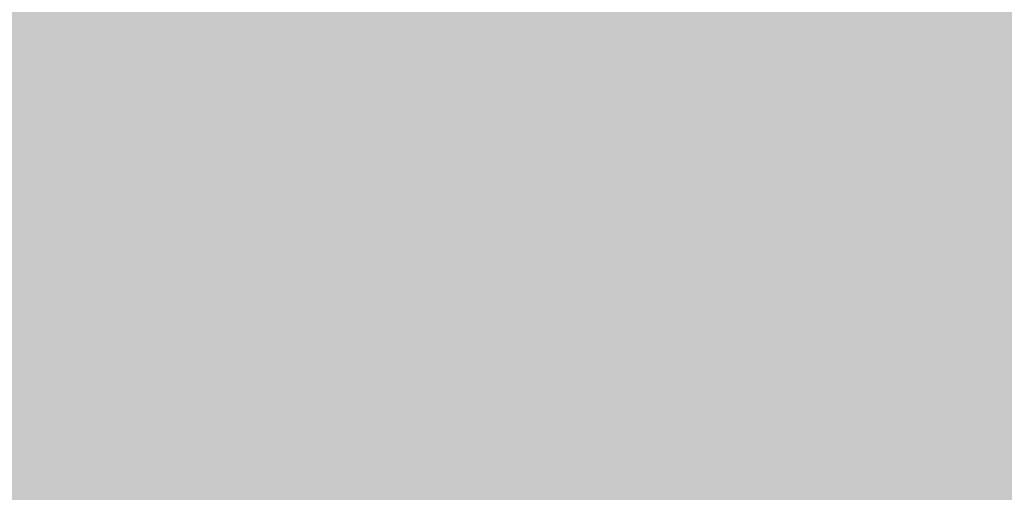
# Model space of a CAD drawing. Units: inches. Extents: x 2083 to 3317, y 1141 to 2115.
# Tile 136 of 256: x 3123.979 to 3126.132, y 1264.131 to 1265.165. Entities that reach past the tile are written whole.
import ezdxf

# ---------------------------------------------------------------- set-up
doc = ezdxf.new("R2010")
doc.units = ezdxf.units.IN
doc.layers.add('A-ANNO-DIMS', color=2, linetype='Continuous', lineweight=18)
doc.layers.add('A-WALL-PATT', color=251, linetype='Continuous', lineweight=13, true_color=0x636466)
doc.styles.get("Standard").update_dxf_attribs({"font": 'arial.ttf'})
doc.dimstyles.new('ISO-25', dxfattribs={"dimtxt": 12, "dimasz": 12, "dimexe": 1.25, "dimexo": 0.625, "dimtad": 1, "dimlunit": 3, "dimtxsty": 'Standard', "dimcen": 2.5, "dimadec": 0, "dimazin": 0, "dimtfac": 1, "dimtmove": 0, "dimatfit": 3, "dimfxl": 1, "dimarcsym": 0})

# ---------------------------------------------------------------- blocks, each defined once
blk = doc.blocks.new('*D26')
at = {"layer": 'A-ANNO-DIMS', "color": 0, "lineweight": -2, "transparency": 16777216}
for p, q in [((3088.9858, 1274.9151), (3088.9858, 1270.952)), ((3111.24, 1274.9151), (3111.24, 1270.952)), ((3076.9858, 1272.202), (2840.2624, 1272.202)), ((3111.24, 1272.202), (3088.9858, 1272.202)), ((3123.24, 1272.202), (3135.24, 1272.202))]:
    blk.add_line(p, q, dxfattribs=at)
at = {"layer": 'A-ANNO-DIMS', "color": 0, "transparency": 16777216}
for points in [[(3076.9858, 1274.202), (3076.9858, 1270.202), (3088.9858, 1272.202)], [(3123.24, 1274.202), (3123.24, 1270.202), (3111.24, 1272.202)]]:
    blk.add_solid(points, dxfattribs=at)
at = {"layer": 'Defpoints', "color": 0, "transparency": 16777216}
for p in [(3088.9858, 1275.5401), (3111.24, 1275.5401), (3088.9858, 1272.202)]:
    blk.add_point(p, dxfattribs=at)
at = {"layer": 'A-ANNO-DIMS', "color": 0, "transparency": 16777216, "insert": (2952.6241, 1279.0316), "char_height": 12, "attachment_point": 5}
blk.add_mtext('NIGHTSTAND 1\'-10 1/2" TYP.', dxfattribs=at)
blk = doc.blocks.new('*D27')
at = {"layer": 'A-ANNO-DIMS', "color": 0, "lineweight": -2, "transparency": 16777216}
for p, q in [((3114.5782, 1309.7943), (3114.5782, 1321.7943)), ((3111.865, 1297.7943), (3115.8282, 1297.7943)), ((3114.5782, 1297.7943), (3114.5782, 1275.5401)), ((3111.865, 1275.5401), (3115.8282, 1275.5401)), ((3114.5782, 1263.5401), (3114.5782, 1140.9886))]:
    blk.add_line(p, q, dxfattribs=at)
at = {"layer": 'A-ANNO-DIMS', "color": 0, "transparency": 16777216}
for points in [[(3112.5782, 1309.7943), (3116.5782, 1309.7943), (3114.5782, 1297.7943)], [(3112.5782, 1263.5401), (3116.5782, 1263.5401), (3114.5782, 1275.5401)]]:
    blk.add_solid(points, dxfattribs=at)
at = {"layer": 'Defpoints', "color": 0, "transparency": 16777216}
for p in [(3111.24, 1297.7943), (3111.24, 1275.5401), (3114.5782, 1275.5401)]:
    blk.add_point(p, dxfattribs=at)
at = {"layer": 'A-ANNO-DIMS', "color": 0, "transparency": 16777216, "insert": (3107.7485, 1196.2643), "char_height": 12, "attachment_point": 5, "rotation": 90}
blk.add_mtext('1\'-10 1/2" TYP.', dxfattribs=at)

msp = doc.modelspace()

# ---------------------------------------------------------------- hatches: boundary and pattern name
at = {"layer": 'A-WALL-PATT'}
h = msp.add_hatch(color=256, dxfattribs=at)
h.dxf.hatch_style = 1
h.paths.add_polyline_path([(3126.9598, 2020.7614), (2748.9598, 2020.7614), (2604.9598, 2020.7614), (2226.9598, 2020.7614), (2226.9598, 1702.7614), (2466.9598, 1702.7614), (2466.9598, 1582.7614), (2418.9598, 1582.7614), (2418.9598, 1477.7614), (2226.9598, 1477.7614), (2226.9598, 1263.2614), (2544.9598, 1263.2614), (2544.9598, 1411.7614), (2604.9598, 1411.7614), (2685.9598, 1411.7614), (2685.9598, 1420.7614), (2604.9598, 1420.7614), (2604.9598, 1573.7614), (2604.9598, 1702.7614), (2604.9598, 2011.7614), (2748.9598, 2011.7614), (2748.9598, 1702.7614), (2862.9598, 1702.7614), (2862.9598, 1621.7614), (2871.9598, 1621.7614), (2871.9598, 1702.7614), (2883.9598, 1702.7614), (2883.9598, 1706.9395, -0.026459), (2883.9598, 1711.7614), (2757.9598, 1711.7614), (2757.9598, 1807.7614), (2787.9598, 1807.7614), (2787.9598, 1812.2614), (2757.9598, 1812.2614), (2757.9598, 2011.7614), (2877.9598, 2011.7614), (2877.9598, 1812.2614), (2847.9598, 1812.2614), (2847.9598, 1807.7614), (2889.8357, 1807.7614), (2889.8357, 1812.2614), (2882.4598, 1812.2614), (2882.4598, 2011.7614), (3117.9598, 2011.7614), (3117.9598, 1812.2614), (2937.8357, 1812.2614), (2937.8357, 1807.7614), (2995.7098, 1807.7614), (2995.7098, 1796.1177), (3000.2098, 1796.1177), (3000.2098, 1807.7614), (3117.9598, 1807.7614), (3117.9598, 1711.7614), (3000.2098, 1711.7614), (3000.2098, 1760.1177), (2998.5727, 1760.1177, -0.020711), (2995.7098, 1760.1177), (2995.7098, 1711.7614), (2931.9598, 1711.7614), (2931.9598, 1702.7614), (3126.9598, 1702.7614)])
h.paths.add_polyline_path([(2471.4598, 2011.7614), (2471.4598, 1810.0114), (2462.7169, 1810.0114), (2462.7169, 1805.5114), (2505.9598, 1805.5114), (2505.9598, 1810.0114), (2475.9598, 1810.0114), (2475.9598, 2011.7614), (2595.9598, 2011.7614), (2595.9598, 1810.0114), (2565.9598, 1810.0114), (2565.9598, 1805.5114), (2595.9598, 1805.5114), (2595.9598, 1711.7614), (2235.9598, 1711.7614), (2235.9598, 1805.5114), (2353.7098, 1805.5114), (2353.7098, 1796.0542), (2358.2098, 1796.0542), (2358.2098, 1805.5114), (2414.7169, 1805.5114), (2414.7169, 1810.0114), (2235.9598, 1810.0114), (2235.9598, 2011.7614)], flags=16)
h.paths.add_polyline_path([(2270.2047, 1994.61), (2270.2047, 1970.61), (2246.2047, 1970.61), (2246.2047, 1994.61)], flags=0)
edge = h.paths.add_edge_path(flags=0)
edge.add_ellipse((2332.0274, 1899.7982), major_axis=(-3.043, 3.043), ratio=0.168252, start_angle=-161.3322, end_angle=-156.3071, ccw=False)
edge.add_ellipse((2333.082, 1898.7435), major_axis=(-1.0546, 1.0546), ratio=0.453532, start_angle=-123.371, end_angle=-94.1591)
edge = h.paths.add_edge_path(flags=0)
edge.add_ellipse((2332.0274, 1968.8763), major_axis=(3.043, 3.043), ratio=0.168252, start_angle=18.6678, end_angle=23.6929)
edge.add_spline(control_points=[(2332.9256, 1970.6911), (2332.2268, 1970.3361), (2330.8937, 1969.6589), (2328.4131, 1970.9321), (2327.2039, 1967.7487), (2324.7096, 1969.9556), (2322.5328, 1967.0124), (2320.0128, 1971.2958), (2317.6803, 1968.1578), (2316.0405, 1967.102), (2315.4269, 1966.8096)], knot_values=[0, 0, 0, 0, 2.267059, 4.324559, 6.685584, 8.878641, 11.121502, 14.300359, 17.755284, 19.732645, 19.732645, 19.732645, 19.732645], degree=3, periodic=0)
edge.add_ellipse((2332.0274, 1968.8763), major_axis=(3.043, 3.043), ratio=0.168252, start_angle=18.6678, end_angle=23.6929, ccw=False)
edge.add_ellipse((2333.082, 1969.9309), major_axis=(1.0546, 1.0546), ratio=0.453532, start_angle=56.629, end_angle=85.8409, ccw=False)
edge = h.paths.add_edge_path(flags=0)
edge.add_spline(control_points=[(2296.4283, 1967.9879), (2293.6278, 1965.3363), (2287.7036, 1959.7271), (2299.7439, 1949.9957), (2294.5326, 1935.6685), (2290.5732, 1920.6035), (2293.3941, 1909.9737), (2296.1854, 1904.9665)], knot_values=[0.099185, 0.099185, 0.099185, 0.099185, 0.345301, 0.619822, 0.982653, 1.386093, 1.810555, 1.810555, 1.810555, 1.810555], degree=3, periodic=0)
edge.add_spline(control_points=[(2296.1854, 1904.9665), (2297.3836, 1902.6193), (2298.001, 1901.9493), (2298.553, 1901.4682)], knot_values=[0.006246, 0.006246, 0.006246, 0.006246, 0.055476, 0.055476, 0.055476, 0.055476], degree=3, periodic=0)
edge.add_spline(control_points=[(2298.553, 1901.4682), (2297.2586, 1900.9232), (2295.2253, 1900.2321), (2293.0602, 1900.6142), (2292.1014, 1900.7884), (2292.0896, 1900.7906)], knot_values=[0.312835, 0.312835, 0.312835, 0.312835, 0.40178, 0.474987, 0.475903, 0.475903, 0.475903, 0.475903], degree=3, periodic=0)
edge.add_arc((2292.7936, 1904.6641), 3.937, 215.4209, 259.6982, ccw=False)
edge.add_spline(control_points=[(2289.5853, 1902.3823), (2289.4767, 1902.5351), (2289.3685, 1902.688), (2289.2609, 1902.8412)], knot_values=[0.102872, 0.102872, 0.102872, 0.102872, 0.116896, 0.116896, 0.116896, 0.116896], degree=3, periodic=0)
edge.add_spline(control_points=[(2289.2609, 1902.8412), (2288.6866, 1902.5502), (2287.64, 1902.0199), (2285.8813, 1901.874), (2283.853, 1901.5044), (2281.72, 1899.7105), (2278.467, 1899.4929), (2276.1571, 1901.8832), (2272.259, 1899.8041), (2267.7776, 1901.8432), (2262.2439, 1900.184), (2257.4149, 1901.7821), (2254.3184, 1900.7261), (2253.1783, 1900.3373)], knot_values=[0, 0, 0, 0, 1.907977, 3.477176, 5.261074, 7.972851, 11.680248, 13.717921, 16.939592, 22.789562, 27.502503, 33.595215, 37.145618, 37.145618, 37.145618, 37.145618], degree=3, periodic=0)
edge.add_line((2253.1783, 1900.3373), (2250.2442, 1902.8412))
edge.add_line((2250.2442, 1902.8412), (2250.2442, 1965.8333))
edge.add_line((2250.2442, 1965.8333), (2253.1783, 1968.3371))
edge.add_spline(control_points=[(2253.1783, 1968.3371), (2254.3184, 1967.9483), (2257.4149, 1966.8924), (2262.2439, 1968.4904), (2267.7776, 1966.8313), (2271.5267, 1968.5372), (2273.8759, 1967.8283), (2274.2067, 1967.7276)], knot_values=[0, 0, 0, 0, 0.09018, 0.244935, 0.364644, 0.513233, 0.537855, 0.537855, 0.537855, 0.537855], degree=3, periodic=0)
edge.add_arc((2274.3529, 1963.7933), 3.937, 72.0511, 92.1279, ccw=False)
edge.add_arc((2281.2969, 1985.23), 18.5963, 252.05113, 288.56572)
edge.add_arc((2292.3167, 1956.0289), 12.6461, 71.02679, 113.77822, ccw=False)
edge = h.paths.add_edge_path(flags=0)
edge.add_spline(control_points=[(2274.8994, 1951.8562), (2275.0662, 1951.6166), (2275.2327, 1951.3766), (2275.398, 1951.1359)], knot_values=[1.409916, 1.409916, 1.409916, 1.409916, 1.43159, 1.43159, 1.43159, 1.43159], degree=3, periodic=0)
edge.add_spline(control_points=[(2275.398, 1951.1359), (2275.7921, 1950.5619), (2276.1792, 1949.9838), (2276.5455, 1949.3971)], knot_values=[1.358238, 1.358238, 1.358238, 1.358238, 1.409916, 1.409916, 1.409916, 1.409916], degree=3, periodic=0)
edge.add_line((2276.5455, 1949.3971), (2277.4373, 1947.8622))
edge.add_spline(control_points=[(2277.4373, 1947.8622), (2276.3038, 1945.6731), (2274.6397, 1942.4269), (2274.6316, 1938.0939), (2272.7991, 1930.8515), (2274.3564, 1943.897), (2275.9477, 1947.9234), (2276.5455, 1949.3971)], knot_values=[0.005632, 0.005632, 0.005632, 0.005632, 0.186014, 0.266002, 0.357087, 0.59639, 0.739732, 0.739732, 0.739732, 0.739732], degree=3, periodic=0)
edge.add_spline(control_points=[(2276.5455, 1949.3971), (2276.1792, 1949.9838), (2275.7921, 1950.5619), (2275.398, 1951.1359)], knot_values=[1.358238, 1.358238, 1.358238, 1.358238, 1.409916, 1.409916, 1.409916, 1.409916], degree=3, periodic=0)
edge.add_spline(control_points=[(2275.398, 1951.1359), (2274.9425, 1950.0805), (2274.2078, 1948.0253), (2273.9346, 1944.8515), (2272.4685, 1937.6275), (2273.4662, 1945.6965), (2274.7006, 1951.0595), (2274.8994, 1951.8562)], knot_values=[0.104364, 0.104364, 0.104364, 0.104364, 0.189636, 0.269624, 0.36071, 0.600013, 0.644622, 0.644622, 0.644622, 0.644622], degree=3, periodic=0)
h.paths.add_polyline_path([(2269.1675, 1963.1276, -0.357527), (2268.1706, 1960.9764, -0.092561), (2268.1706, 1939.4363, -0.357527), (2269.1675, 1937.2851, -0.357527), (2267.0163, 1938.282, -0.164785), (2254.6856, 1938.282, -0.357527), (2252.5344, 1937.2851, -0.357527), (2253.5313, 1939.4363, -0.092561), (2253.5313, 1960.9764, -0.357527), (2252.5344, 1963.1276, -0.357527), (2254.6856, 1962.1307, -0.164785), (2267.0163, 1962.1307, -0.357527)], flags=0)
h.paths.add_polyline_path([(2248.8741, 1967.8018), (2248.8741, 1957.0277), (2249.4578, 1957.0277), (2249.4578, 1911.6468), (2248.8741, 1911.6468), (2248.8741, 1900.8727), (2246.5119, 1900.8727, 0.197327), (2244.1497, 1902.4569), (2244.1497, 1966.2176, 0.197327), (2246.5119, 1967.8018)], flags=0)
h.paths.add_polyline_path([(2269.1675, 1931.3893, -0.357527), (2268.1706, 1929.2381, -0.092561), (2268.1706, 1907.6981, -0.357527), (2269.1675, 1905.5469, -0.357527), (2267.0163, 1906.5438, -0.164785), (2254.6856, 1906.5438, -0.357527), (2252.5344, 1905.5469, -0.357527), (2253.5313, 1907.6981, -0.092561), (2253.5313, 1929.2381, -0.357527), (2252.5344, 1931.3893, -0.357527), (2254.6856, 1930.3925, -0.164785), (2267.0163, 1930.3925, -0.357527)], flags=0)
edge = h.paths.add_edge_path(flags=0)
edge.add_spline(control_points=[(2276.1969, 1906.7237), (2276.1681, 1909.0289), (2276.114, 1913.3719), (2270.5984, 1924.925), (2273.9052, 1919.0128), (2275.9217, 1916.2621), (2275.4746, 1912.4021), (2277.2579, 1910.3806), (2276.696, 1908.225), (2276.6462, 1906.813), (2276.6178, 1906.0084)], knot_values=[0, 0, 0, 0, 8.61026, 16.221274, 18.843057, 23.804898, 27.440828, 29.356102, 31.203478, 33.650687, 33.650687, 33.650687, 33.650687], degree=3, periodic=0)
edge.add_spline(control_points=[(2276.6178, 1906.0084), (2276.6233, 1905.6241), (2276.4977, 1904.6287), (2275.4418, 1903.8547), (2274.9373, 1903.0804), (2274.8591, 1902.8412)], knot_values=[0.156488, 0.156488, 0.156488, 0.156488, 0.184398, 0.231376, 0.250598, 0.250598, 0.250598, 0.250598], degree=3, periodic=0)
edge.add_line((2274.8591, 1902.8412), (2276.506, 1902.8412))
edge.add_spline(control_points=[(2276.506, 1902.8412), (2276.7883, 1903.0849), (2277.6651, 1904.1252), (2278.2495, 1904.3407), (2277.6539, 1908.5274), (2278.1557, 1906.2278), (2278.1005, 1905.2859), (2278.8467, 1904.069), (2277.8568, 1903.4149), (2277.8742, 1902.991), (2277.9036, 1902.8412)], knot_values=[0.059574, 0.059574, 0.059574, 0.059574, 0.080753, 0.103741, 0.16972, 0.176036, 0.207137, 0.240474, 0.262341, 0.27366, 0.27366, 0.27366, 0.27366], degree=3, periodic=0)
edge.add_line((2277.9036, 1902.8412), (2280.0298, 1902.8412))
edge.add_spline(control_points=[(2280.0298, 1902.8412), (2279.8882, 1903.0884), (2279.4993, 1903.9816), (2280.1523, 1905.9393), (2278.1036, 1909.6578), (2279.7624, 1907.1853), (2280.3279, 1904.8749), (2280.4851, 1903.4896), (2281.4633, 1903.2494), (2281.7583, 1902.9365), (2281.834, 1902.8412)], knot_values=[0.013856, 0.013856, 0.013856, 0.013856, 0.034874, 0.088867, 0.107879, 0.126738, 0.158714, 0.193757, 0.217487, 0.226722, 0.226722, 0.226722, 0.226722], degree=3, periodic=0)
edge.add_spline(control_points=[(2281.834, 1902.8412), (2281.7875, 1902.8267), (2281.647, 1902.783), (2281.3955, 1902.8595), (2281.0881, 1902.9852), (2280.7207, 1903.0609), (2280.3335, 1903.0257), (2280.1248, 1902.8989), (2280.0298, 1902.8412)], knot_values=[0, 0, 0, 0, 0.14413, 0.435517, 0.749276, 1.153046, 1.548371, 1.878348, 1.878348, 1.878348, 1.878348], degree=3, periodic=0)
edge.add_line((2280.0298, 1902.8412), (2277.9036, 1902.8412))
edge.add_spline(control_points=[(2277.9036, 1902.8412), (2277.8929, 1902.7959), (2277.8654, 1902.6796), (2277.6075, 1902.6875), (2277.2741, 1902.8007), (2276.8379, 1902.6198), (2276.5838, 1902.7893), (2276.506, 1902.8412)], knot_values=[0, 0, 0, 0, 0.127189, 0.326199, 0.628009, 1.24357, 1.515331, 1.515331, 1.515331, 1.515331], degree=3, periodic=0)
edge.add_line((2276.506, 1902.8412), (2274.8591, 1902.8412))
edge.add_spline(control_points=[(2274.8591, 1902.8412), (2274.8144, 1902.8986), (2274.7251, 1903.0134), (2274.4935, 1903.119), (2274.2443, 1902.9605), (2273.9371, 1903.1849), (2273.614, 1902.9831), (2273.4083, 1902.883), (2273.3223, 1902.8412)], knot_values=[0, 0, 0, 0, 0.21843, 0.436957, 0.687977, 0.990379, 1.398396, 1.69185, 1.69185, 1.69185, 1.69185], degree=3, periodic=0)
edge.add_spline(control_points=[(2273.3223, 1902.8412), (2273.6167, 1903.4457), (2274.274, 1904.5383), (2276.0272, 1904.5737), (2276.207, 1906.5836), (2276.1969, 1906.7237)], knot_values=[0.012227, 0.012227, 0.012227, 0.012227, 0.059472, 0.106218, 0.134458, 0.134458, 0.134458, 0.134458], degree=3, periodic=0)
h.paths.add_polyline_path([(2270.7761, 1897.7898), (2270.7761, 1873.7898), (2246.7761, 1873.7898), (2246.7761, 1897.7898)], flags=0)
h.paths.add_polyline_path([(2353.7098, 1760.0051), (2353.7098, 1760.0542), (2358.2098, 1760.0542, -0.033729)], flags=0)
h.paths.add_polyline_path([(2321.8191, 1737.5292), (2341.9953, 1737.5292, -0.414214), (2343.2033, 1736.3212), (2343.2033, 1721.0206, -0.414214), (2341.9953, 1719.8127), (2321.8191, 1719.8127, -0.414214), (2320.6112, 1721.0206), (2320.6112, 1736.3212, -0.414214)], flags=0)
h.paths.add_polyline_path([(2324.235, 1736.3212), (2339.5794, 1736.3212, -0.414214), (2341.9953, 1733.9053), (2341.9953, 1725.4497, -0.414214), (2339.5794, 1723.0338), (2333.6806, 1723.0338), (2333.8453, 1722.0455, -0.870646), (2335.4254, 1721.8259, -0.767327), (2333.9227, 1721.4232), (2331.291, 1721.4232, -0.767327), (2329.7883, 1721.8259, -0.870646), (2331.3684, 1722.0455), (2331.5331, 1723.0338), (2324.235, 1723.0338, -0.414214), (2321.8191, 1725.4497), (2321.8191, 1733.9053, -0.414214)], flags=0)
h.paths.add_polyline_path([(2570.4838, 1928.6154), (2589.6838, 1928.6154), (2590.1688, 1928.6154), (2590.1688, 1904.9934), (2570.4838, 1904.9934)], flags=0)
h.paths.add_polyline_path([(2574.4473, 1927.2638, -1), (2572.8288, 1927.2638, -1)], flags=0)
h.paths.add_polyline_path([(2573.0899, 1926.9409), (2573.925, 1927.776), (2574.1477, 1927.5533), (2573.3126, 1926.7182)], flags=0)
h.paths.add_polyline_path([(2578.7791, 1919.7296, -1), (2571.5917, 1919.7296, -1)], flags=0)
h.paths.add_polyline_path([(2578.3854, 1919.7296, -1), (2571.9854, 1919.7296, -1)], flags=0)
h.paths.add_polyline_path([(2331.5958, 1729.4762, -1), (2333.618, 1729.4762, -1)], flags=0)
h.paths.add_polyline_path([(2578.0342, 1927.2638, -1), (2576.4157, 1927.2638, -1)], flags=0)
h.paths.add_polyline_path([(2576.6889, 1927.5311), (2576.9116, 1927.7538), (2577.7467, 1926.9186), (2577.524, 1926.6959)], flags=0)
h.paths.add_polyline_path([(2578.1391, 1909.8595, -1), (2572.2317, 1909.8595, -1)], flags=0)
h.paths.add_polyline_path([(2577.7454, 1909.8595, -1), (2572.6254, 1909.8595, -1)], flags=0)
h.paths.add_polyline_path([(2583.7977, 1927.2638, -1), (2582.1792, 1927.2638, -1)], flags=0)
h.paths.add_polyline_path([(2582.7186, 1927.7538), (2583.5538, 1926.9186), (2583.3311, 1926.6959), (2582.4959, 1927.5311)], flags=0)
h.paths.add_polyline_path([(2582.4959, 1927.5311), (2582.7186, 1927.7538), (2583.5538, 1926.9186), (2583.3311, 1926.6959)], flags=0)
h.paths.add_polyline_path([(2587.7391, 1920.5296, -1), (2581.8317, 1920.5296, -1)], flags=0)
h.paths.add_polyline_path([(2587.3454, 1920.5296, -1), (2582.2254, 1920.5296, -1)], flags=0)
h.paths.add_polyline_path([(2587.3846, 1927.2638, -1), (2585.7661, 1927.2638, -1)], flags=0)
h.paths.add_polyline_path([(2586.082, 1926.9802), (2586.9172, 1927.8154), (2587.1399, 1927.5927), (2586.3047, 1926.7575)], flags=0)
h.paths.add_polyline_path([(2588.3791, 1910.6595, -1), (2581.1917, 1910.6595, -1)], flags=0)
h.paths.add_polyline_path([(2587.9854, 1910.6595, -1), (2581.5854, 1910.6595, -1)], flags=0)
h.paths.add_polyline_path([(2417.1677, 1729.4779), (2437.3439, 1729.4779, -0.414214), (2438.5519, 1728.2699), (2438.5519, 1712.9693, -0.414214), (2437.3439, 1711.7614), (2417.1677, 1711.7614, -0.414214), (2415.9598, 1712.9693), (2415.9598, 1728.2699, -0.414214)], flags=0)
h.paths.add_polyline_path([(2419.5836, 1728.2699), (2434.928, 1728.2699, -0.414214), (2437.3439, 1725.8541), (2437.3439, 1717.3984, -0.414214), (2434.928, 1714.9825), (2429.0292, 1714.9825), (2429.1939, 1713.9942, -0.870646), (2430.774, 1713.7746, -0.767327), (2429.2713, 1713.372), (2426.6396, 1713.372, -0.767327), (2425.1369, 1713.7746, -0.870646), (2426.717, 1713.9942), (2426.8817, 1714.9825), (2419.5836, 1714.9825, -0.414214), (2417.1677, 1717.3984), (2417.1677, 1725.8541, -0.414214)], flags=0)
h.paths.add_polyline_path([(2419.5836, 1728.2699), (2434.928, 1728.2699, -0.414214), (2437.3439, 1725.8541), (2437.3439, 1717.3984, -0.414214), (2434.928, 1714.9825), (2429.0292, 1714.9825), (2428.3581, 1719.009), (2427.5528, 1719.009), (2426.8817, 1714.9825), (2419.5836, 1714.9825, -0.414214), (2417.1677, 1717.3984), (2417.1677, 1725.8541, -0.414214)], flags=0)
h.paths.add_polyline_path([(2426.9444, 1721.4249, -1), (2428.9666, 1721.4249, -1)], flags=0)
h.paths.add_polyline_path([(2475.9598, 1702.7614), (2595.9598, 1702.7614), (2595.9598, 1582.7614), (2475.9598, 1582.7614)], flags=16)
h.paths.add_polyline_path([(2427.9598, 1573.7614), (2595.9598, 1573.7614), (2595.9598, 1468.7614), (2595.9598, 1420.7614), (2384.4598, 1420.7614), (2384.4598, 1468.7614), (2427.9598, 1468.7614)], flags=16)
h.paths.add_polyline_path([(2379.9598, 1468.7614), (2379.9598, 1420.7614), (2235.9598, 1420.7614), (2235.9598, 1468.7614)], flags=16)
h.paths.add_polyline_path([(2317.816, 1466.6958), (2337.9922, 1466.6958, -0.414214), (2339.2002, 1465.4878), (2339.2002, 1450.1872, -0.414214), (2337.9922, 1448.9792), (2317.816, 1448.9792, -0.414214), (2316.6081, 1450.1872), (2316.6081, 1465.4878, -0.414214)], flags=0)
h.paths.add_polyline_path([(2320.2319, 1465.4878), (2335.5763, 1465.4878, -0.414214), (2337.9922, 1463.0719), (2337.9922, 1454.6163, -0.414214), (2335.5763, 1452.2004), (2329.6775, 1452.2004), (2329.8422, 1451.212, -0.870646), (2331.4223, 1450.9925, -0.767327), (2329.9196, 1450.5898), (2327.2879, 1450.5898, -0.767327), (2325.7852, 1450.9925, -0.870646), (2327.3653, 1451.212), (2327.53, 1452.2004), (2320.2319, 1452.2004, -0.414214), (2317.816, 1454.6163), (2317.816, 1463.0719, -0.414214)], flags=0)
h.paths.add_polyline_path([(2320.2319, 1465.4878), (2335.5763, 1465.4878, -0.414214), (2337.9922, 1463.0719), (2337.9922, 1454.6163, -0.414214), (2335.5763, 1452.2004), (2329.6775, 1452.2004), (2329.0064, 1456.2269), (2328.2011, 1456.2269), (2327.53, 1452.2004), (2320.2319, 1452.2004, -0.414214), (2317.816, 1454.6163), (2317.816, 1463.0719, -0.414214)], flags=0)
h.paths.add_polyline_path([(2327.5926, 1458.6428, -1), (2329.6148, 1458.6428, -1)], flags=0)
h.paths.add_polyline_path([(2244.4117, 1433.3405), (2241.9209, 1433.3405, -0.414214), (2240.0179, 1435.2435), (2240.0179, 1440.9528, -0.414211), (2241.9209, 1442.8559), (2244.4117, 1442.8559, -1.976472)], flags=0)
h.paths.add_polyline_path([(2245.3569, 1434.3975, -0.414214), (2245.3569, 1441.7988, -2.144098)], flags=0)
h.paths.add_polyline_path([(2535.9598, 1416.2614), (2535.9598, 1272.2614), (2235.9598, 1272.2614), (2235.9598, 1416.2614)], flags=16)
h.paths.add_polyline_path([(2260.1196, 1384.2928), (2260.1196, 1362.0386), (2237.8654, 1362.0386), (2237.8654, 1384.2928)], flags=0)
edge = h.paths.add_edge_path(flags=0)
edge.add_line((2318.2518, 1362.0933), (2318.1458, 1362.001))
edge.add_ellipse((2317.4451, 1360.431), major_axis=(2.8216, 2.8216), ratio=0.168252, start_angle=18.6678, end_angle=20.9481, ccw=False)
edge.add_ellipse((2318.423, 1361.409), major_axis=(0.9779, 0.9779), ratio=0.453532, start_angle=56.629, end_angle=70.2262, ccw=False)
edge = h.paths.add_edge_path(flags=0)
edge.add_line((2319.1074, 1295.5711), (2319.015, 1295.6771))
edge.add_ellipse((2317.4451, 1296.3778), major_axis=(-2.8216, 2.8216), ratio=0.168252, start_angle=-161.3322, end_angle=-159.0519, ccw=False)
edge.add_ellipse((2318.423, 1295.3999), major_axis=(-0.9779, 0.9779), ratio=0.453532, start_angle=-123.371, end_angle=-109.7738)
edge = h.paths.add_edge_path(flags=0)
edge.add_spline(control_points=[(2284.2103, 1301.1702), (2284.5807, 1300.4447), (2284.8912, 1299.892), (2285.1596, 1299.461)], knot_values=[0.039066, 0.039066, 0.039066, 0.039066, 0.055476, 0.055476, 0.055476, 0.055476], degree=3, periodic=0)
edge.add_line((2285.1596, 1299.461), (2284.2103, 1301.1702))
edge = h.paths.add_edge_path(flags=0)
edge.add_line((2280.4125, 1297.298), (2283.37, 1297.0361))
edge.add_line((2283.37, 1297.0361), (2286.4057, 1297.9263))
edge.add_spline(control_points=[(2286.4057, 1297.9263), (2285.3055, 1297.4631), (2284.3448, 1297.1292), (2283.37, 1297.0361)], knot_values=[0.394369, 0.394369, 0.394369, 0.394369, 0.475903, 0.475903, 0.475903, 0.475903], degree=3, periodic=0)
edge.add_spline(control_points=[(2283.37, 1297.0361), (2283.2814, 1297.0277), (2282.3163, 1296.9573), (2281.3125, 1297.1345), (2280.4234, 1297.296), (2280.4125, 1297.298)], knot_values=[0.312835, 0.312835, 0.312835, 0.312835, 0.320246, 0.393453, 0.394369, 0.394369, 0.394369, 0.394369], degree=3, periodic=0)
edge = h.paths.add_edge_path(flags=0)
edge.add_line((2284.4356, 1359.6073), (2280.4463, 1355.328))
edge.add_line((2280.4463, 1355.328), (2279.58, 1351.0178))
edge.add_line((2279.58, 1351.0178), (2282.413, 1346.5804))
edge.add_spline(control_points=[(2282.413, 1346.5804), (2283.1533, 1345.5892), (2284.2529, 1344.0289), (2284.801, 1342.3872), (2284.9352, 1341.8055)], knot_values=[1.240098, 1.240098, 1.240098, 1.240098, 1.332892, 1.382712, 1.382712, 1.382712, 1.382712], degree=3, periodic=0)
edge.add_spline(control_points=[(2284.9352, 1341.8055), (2285.3191, 1340.1406), (2285.233, 1338.4092), (2284.9099, 1336.6541)], knot_values=[1.097484, 1.097484, 1.097484, 1.097484, 1.240098, 1.240098, 1.240098, 1.240098], degree=3, periodic=0)
edge.add_spline(control_points=[(2284.9099, 1336.6541), (2284.5868, 1334.899), (2284.0267, 1333.1203), (2283.4626, 1331.3606)], knot_values=[0.95487, 0.95487, 0.95487, 0.95487, 1.097484, 1.097484, 1.097484, 1.097484], degree=3, periodic=0)
edge.add_line((2283.4626, 1331.3606), (2281.8904, 1326.1534))
edge.add_line((2281.8904, 1326.1534), (2280.7563, 1321.0561))
edge.add_line((2280.7563, 1321.0561), (2280.2992, 1316.002))
edge.add_line((2280.2992, 1316.002), (2280.7159, 1310.9501))
edge.add_line((2280.7159, 1310.9501), (2282.0281, 1305.9721))
edge.add_line((2282.0281, 1305.9721), (2284.2103, 1301.1702))
edge.add_spline(control_points=[(2284.2103, 1301.1702), (2283.3407, 1302.7302), (2282.6119, 1304.3365), (2282.0281, 1305.9721)], knot_values=[0.099185, 0.099185, 0.099185, 0.099185, 0.241799, 0.241799, 0.241799, 0.241799], degree=3, periodic=0)
edge.add_spline(control_points=[(2282.0281, 1305.9721), (2281.4443, 1307.6078), (2281.0055, 1309.2728), (2280.7159, 1310.9501)], knot_values=[0.241799, 0.241799, 0.241799, 0.241799, 0.384413, 0.384413, 0.384413, 0.384413], degree=3, periodic=0)
edge.add_spline(control_points=[(2280.7159, 1310.9501), (2280.4332, 1312.5876), (2280.2894, 1314.277), (2280.2989, 1315.962), (2280.2992, 1316.002)], knot_values=[0.384413, 0.384413, 0.384413, 0.384413, 0.523647, 0.527028, 0.527028, 0.527028, 0.527028], degree=3, periodic=0)
edge.add_spline(control_points=[(2280.2992, 1316.002), (2280.3123, 1317.687), (2280.4779, 1319.3679), (2280.7563, 1321.0561)], knot_values=[0.527028, 0.527028, 0.527028, 0.527028, 0.669642, 0.669642, 0.669642, 0.669642], degree=3, periodic=0)
edge.add_spline(control_points=[(2280.7563, 1321.0561), (2281.0346, 1322.7443), (2281.4259, 1324.4396), (2281.8904, 1326.1534)], knot_values=[0.669642, 0.669642, 0.669642, 0.669642, 0.812256, 0.812256, 0.812256, 0.812256], degree=3, periodic=0)
edge.add_spline(control_points=[(2281.8904, 1326.1534), (2282.2644, 1327.5333), (2282.7879, 1329.2618), (2283.3528, 1331.0178), (2283.4626, 1331.3606)], knot_values=[0.812256, 0.812256, 0.812256, 0.812256, 0.927087, 0.95487, 0.95487, 0.95487, 0.95487], degree=3, periodic=0)
edge.add_line((2283.4626, 1331.3606), (2284.9099, 1336.6541))
edge.add_line((2284.9099, 1336.6541), (2284.9352, 1341.8055))
edge.add_line((2284.9352, 1341.8055), (2282.413, 1346.5804))
edge.add_spline(control_points=[(2282.413, 1346.5804), (2281.2751, 1348.1038), (2280.0784, 1349.5703), (2279.58, 1351.0178)], knot_values=[1.382712, 1.382712, 1.382712, 1.382712, 1.525326, 1.525326, 1.525326, 1.525326], degree=3, periodic=0)
edge.add_spline(control_points=[(2279.58, 1351.0178), (2279.4433, 1351.4147), (2279.1363, 1352.8569), (2279.7352, 1354.2904), (2280.4463, 1355.328)], knot_values=[1.525326, 1.525326, 1.525326, 1.525326, 1.564439, 1.667941, 1.667941, 1.667941, 1.667941], degree=3, periodic=0)
edge.add_spline(control_points=[(2280.4463, 1355.328), (2281.4261, 1356.7578), (2282.9308, 1358.1826), (2284.4356, 1359.6073)], knot_values=[1.667941, 1.667941, 1.667941, 1.667941, 1.810555, 1.810555, 1.810555, 1.810555], degree=3, periodic=0)
edge.add_arc((2280.6231, 1348.5182), 11.7262, 71.02679, 113.77822)
edge.add_arc((2270.4049, 1375.5952), 17.2436, 252.05113, 288.56572, ccw=False)
edge.add_arc((2263.966, 1355.7178), 3.6506, 72.0511, 92.1279)
edge.add_arc((2263.966, 1355.7178), 3.6506, 92.1279, 177.9851)
edge.add_spline(control_points=[(2260.3176, 1355.8462), (2260.2604, 1354.2207), (2260.5513, 1350.1865), (2262.9993, 1346.7663), (2264.4727, 1344.649)], knot_values=[1.43159, 1.43159, 1.43159, 1.43159, 1.564144, 1.770695, 1.770695, 1.770695, 1.770695], degree=3, periodic=0)
edge.add_line((2264.4727, 1344.649), (2264.9356, 1343.9825))
edge.add_spline(control_points=[(2263.801, 1340.2481), (2263.8432, 1340.5141), (2264.0672, 1341.7565), (2264.5127, 1343.0025), (2264.935, 1343.9811)], knot_values=[0.53657, 0.53657, 0.53657, 0.53657, 0.559349, 0.644622, 0.644622, 0.644622, 0.644622], degree=3, periodic=0)
edge.add_spline(control_points=[(2264.935, 1343.9811), (2265.1178, 1343.715), (2265.2989, 1343.4479), (2265.4768, 1343.1794)], knot_values=[1.384077, 1.384077, 1.384077, 1.384077, 1.409916, 1.409916, 1.409916, 1.409916], degree=3, periodic=0)
edge.add_spline(control_points=[(2265.4768, 1343.1794), (2265.6546, 1342.9108), (2265.8293, 1342.6408), (2265.9991, 1342.3688)], knot_values=[1.358238, 1.358238, 1.358238, 1.358238, 1.384077, 1.384077, 1.384077, 1.384077], degree=3, periodic=0)
edge.add_line((2265.9991, 1342.3688), (2266.826, 1340.9455))
edge.add_spline(control_points=[(2266.826, 1340.9455), (2268.8944, 1337.0897), (2271.3982, 1325.843), (2270.5162, 1310.5686), (2275.9194, 1301.8606), (2277.7895, 1299.1994)], knot_values=[0.116896, 0.116896, 0.116896, 0.116896, 0.472987, 1.050969, 1.313793, 1.313793, 1.313793, 1.313793], degree=3, periodic=0)
edge.add_spline(control_points=[(2277.7895, 1299.1994), (2277.8394, 1299.1285), (2277.8894, 1299.0575), (2277.9396, 1298.9866)], knot_values=[0.109884, 0.109884, 0.109884, 0.109884, 0.116896, 0.116896, 0.116896, 0.116896], degree=3, periodic=0)
edge.add_line((2277.9396, 1298.9866), (2277.7888, 1299.1991))
edge.add_spline(control_points=[(2277.7888, 1299.1991), (2277.2566, 1298.9294), (2276.2864, 1298.4379), (2275.0394, 1298.3344), (2274.3833, 1298.2389), (2274.2153, 1298.2093)], knot_values=[33.12187, 33.12187, 33.12187, 33.12187, 35.029056, 36.598255, 37.144827, 37.144827, 37.144827, 37.144827], degree=3, periodic=0)
edge.add_line((2274.2153, 1298.2093), (2273.0731, 1297.893))
edge.add_spline(control_points=[(2273.0731, 1297.893), (2272.3229, 1297.5798), (2271.0392, 1296.5105), (2269.2484, 1296.2261), (2268.4231, 1296.3747)], knot_values=[26.532584, 26.532584, 26.532584, 26.532584, 29.198919, 31.839101, 31.839101, 31.839101, 31.839101], degree=3, periodic=0)
edge.add_line((2268.4231, 1296.3747), (2263.8785, 1297.4575))
edge.add_spline(control_points=[(2263.8785, 1297.4575), (2263.5561, 1297.3594), (2261.8603, 1296.8387), (2260.2388, 1297.2824), (2258.9335, 1297.5165)], knot_values=[15.919551, 15.919551, 15.919551, 15.919551, 16.939592, 21.226067, 21.226067, 21.226067, 21.226067], degree=3, periodic=0)
edge.add_line((2258.9335, 1297.5165), (2254.0552, 1297.329))
edge.add_spline(control_points=[(2254.0552, 1297.329), (2253.7555, 1297.2958), (2252.1137, 1297.1652), (2250.4619, 1297.5442), (2249.1297, 1297.6679)], knot_values=[5.306517, 5.306517, 5.306517, 5.306517, 6.276435, 10.613034, 10.613034, 10.613034, 10.613034], degree=3, periodic=0)
edge.add_line((2249.1297, 1297.6679), (2244.3316, 1296.8778))
edge.add_line((2244.3316, 1296.8778), (2241.611, 1299.1994))
edge.add_line((2241.611, 1299.1994), (2241.611, 1357.6094))
edge.add_line((2241.611, 1357.6094), (2244.3316, 1359.9311))
edge.add_line((2244.3316, 1359.9311), (2252.7288, 1359.5427))
edge.add_spline(control_points=[(2252.7288, 1359.5427), (2252.8709, 1359.5464), (2253.3057, 1359.5482), (2253.7398, 1359.5143), (2254.0317, 1359.4824)], knot_values=[0.233291, 0.233291, 0.233291, 0.233291, 0.244935, 0.268927, 0.268927, 0.268927, 0.268927], degree=3, periodic=0)
edge.add_line((2254.0317, 1359.4824), (2259.5872, 1359.4164))
edge.add_spline(control_points=[(2259.5872, 1359.4164), (2260.6771, 1359.6285), (2262.0732, 1359.897), (2263.5237, 1359.4593), (2263.8304, 1359.366)], knot_values=[0.422516, 0.422516, 0.422516, 0.422516, 0.513233, 0.537855, 0.537855, 0.537855, 0.537855], degree=3, periodic=0)
edge.add_arc((2263.966, 1355.7178), 3.6506, 72.0511, 92.1279, ccw=False)
edge.add_arc((2270.4049, 1375.5952), 17.2436, 252.05113, 288.56572)
edge.add_arc((2280.6231, 1348.5182), 11.7262, 71.02679, 113.77822, ccw=False)
h.paths.add_polyline_path([(2240.3405, 1359.4347), (2240.3405, 1349.4444), (2240.8818, 1349.4444), (2240.8818, 1307.3645), (2240.3405, 1307.3645), (2240.3405, 1297.3741), (2238.1502, 1297.3741, 0.197327), (2235.9598, 1298.8431), (2235.9598, 1357.9657, 0.197327), (2238.1502, 1359.4347)], flags=0)
h.paths.add_polyline_path([(2259.1578, 1355.1005, -0.357527), (2258.2334, 1353.1058, -0.092561), (2258.2334, 1333.1326, -0.357527), (2259.1578, 1331.1379, -0.357527), (2257.1631, 1332.0622, -0.164785), (2245.7293, 1332.0622, -0.357527), (2243.7346, 1331.1379, -0.357527), (2244.6589, 1333.1326, -0.092561), (2244.6589, 1353.1058, -0.357527), (2243.7346, 1355.1005, -0.357527), (2245.7293, 1354.1761, -0.164785), (2257.1631, 1354.1761, -0.357527)], flags=0)
edge = h.paths.add_edge_path(flags=0)
edge.add_line((2265.9991, 1342.3688), (2266.826, 1340.9455))
edge.add_line((2266.826, 1340.9455), (2265.3076, 1337.8141))
edge.add_line((2265.3076, 1337.8141), (2264.3582, 1334.6529))
edge.add_line((2264.3582, 1334.6529), (2264.262, 1333.7997))
edge.add_spline(control_points=[(2264.262, 1333.7997), (2264.2084, 1333.1871), (2264.1621, 1332.3655), (2264.0071, 1331.4139), (2263.969, 1331.2018)], knot_values=[0.464444, 0.464444, 0.464444, 0.464444, 0.516691, 0.531608, 0.531608, 0.531608, 0.531608], degree=3, periodic=0)
edge.add_spline(control_points=[(2263.969, 1331.2018), (2263.7745, 1330.1189), (2263.4244, 1328.7908), (2263.2574, 1328.5307), (2263.234, 1328.5146)], knot_values=[0.372682, 0.372682, 0.372682, 0.372682, 0.44885, 0.464444, 0.464444, 0.464444, 0.464444], degree=3, periodic=0)
edge.add_spline(control_points=[(2263.234, 1328.5146), (2263.0964, 1328.4202), (2263.1312, 1329.3015), (2263.275, 1330.6157)], knot_values=[0.280919, 0.280919, 0.280919, 0.280919, 0.372682, 0.372682, 0.372682, 0.372682], degree=3, periodic=0)
edge.add_spline(control_points=[(2263.275, 1330.6157), (2263.4187, 1331.93), (2263.6715, 1333.6773), (2263.9699, 1335.315)], knot_values=[0.189157, 0.189157, 0.189157, 0.189157, 0.280919, 0.280919, 0.280919, 0.280919], degree=3, periodic=0)
edge.add_spline(control_points=[(2263.9699, 1335.315), (2264.1005, 1336.0322), (2264.4188, 1337.6219), (2264.7548, 1338.8644), (2264.9474, 1339.4911)], knot_values=[0.097394, 0.097394, 0.097394, 0.097394, 0.137578, 0.189157, 0.189157, 0.189157, 0.189157], degree=3, periodic=0)
edge.add_spline(control_points=[(2264.9474, 1339.4911), (2265.29, 1340.6061), (2265.6442, 1341.494), (2265.9991, 1342.3688)], knot_values=[0.005632, 0.005632, 0.005632, 0.005632, 0.097394, 0.097394, 0.097394, 0.097394], degree=3, periodic=0)
h.paths.add_polyline_path([(2259.1578, 1325.671, -0.357527), (2258.2334, 1323.6763, -0.092561), (2258.2334, 1303.7031, -0.357527), (2259.1578, 1301.7084, -0.357527), (2257.1631, 1302.6327, -0.164785), (2245.7293, 1302.6327, -0.357527), (2243.7346, 1301.7084, -0.357527), (2244.6589, 1303.7031, -0.092561), (2244.6589, 1323.6763, -0.357527), (2243.7346, 1325.671, -0.357527), (2245.7293, 1324.7466, -0.164785), (2257.1631, 1324.7466, -0.357527)], flags=0)
edge = h.paths.add_edge_path(flags=0)
edge.add_spline(control_points=[(2261.7089, 1317.3114), (2261.6795, 1317.4176), (2261.7619, 1317.3885), (2262.4907, 1316.0899), (2262.9622, 1315.3009)], knot_values=[14.955861, 14.955861, 14.955861, 14.955861, 16.221274, 18.694826, 18.694826, 18.694826, 18.694826], degree=3, periodic=0)
edge.add_spline(control_points=[(2262.9622, 1315.3009), (2262.9904, 1315.2536), (2263.7021, 1314.0674), (2264.349, 1313.1272), (2264.7301, 1312.1642)], knot_values=[18.694826, 18.694826, 18.694826, 18.694826, 18.843057, 22.433791, 22.433791, 22.433791, 22.433791], degree=3, periodic=0)
edge.add_spline(control_points=[(2264.7301, 1312.1642), (2264.8756, 1311.7964), (2265.1769, 1310.7698), (2265.1431, 1309.5593), (2265.2477, 1308.8242)], knot_values=[22.433791, 22.433791, 22.433791, 22.433791, 23.804898, 26.172756, 26.172756, 26.172756, 26.172756], degree=3, periodic=0)
edge.add_line((2265.2477, 1308.8242), (2265.8508, 1307.1719))
edge.add_spline(control_points=[(2265.8508, 1307.1719), (2266.065, 1306.8217), (2266.3844, 1306.3322), (2266.4244, 1305.7805), (2266.4204, 1305.6112)], knot_values=[28.062562, 28.062562, 28.062562, 28.062562, 29.356102, 29.911721, 29.911721, 29.911721, 29.911721], degree=3, periodic=0)
edge.add_spline(control_points=[(2266.4204, 1305.6112), (2266.4161, 1305.4326), (2266.394, 1305.25), (2266.3648, 1305.0659)], knot_values=[29.911721, 29.911721, 29.911721, 29.911721, 30.497837, 30.497837, 30.497837, 30.497837], degree=3, periodic=0)
edge.add_line((2266.3648, 1305.0659), (2266.0662, 1302.1363))
edge.add_spline(control_points=[(2266.0662, 1302.1363), (2266.0712, 1301.78), (2265.9981, 1301.2), (2265.6633, 1300.759), (2265.5089, 1300.5859)], knot_values=[0.156488, 0.156488, 0.156488, 0.156488, 0.184398, 0.203543, 0.203543, 0.203543, 0.203543], degree=3, periodic=0)
edge.add_line((2265.5089, 1300.5859), (2264.4353, 1299.1994))
edge.add_line((2264.4353, 1299.1994), (2265.9624, 1299.1994))
edge.add_line((2265.9624, 1299.1994), (2267.336, 1301.1753))
edge.add_line((2267.336, 1301.1753), (2267.3117, 1301.9862))
edge.add_spline(control_points=[(2267.3117, 1301.9862), (2267.2611, 1302.8624), (2267.1602, 1303.7371), (2267.2715, 1303.3259)], knot_values=[0.126229, 0.126229, 0.126229, 0.126229, 0.166617, 0.166617, 0.166617, 0.166617], degree=3, periodic=0)
edge.add_spline(control_points=[(2267.2715, 1303.3259), (2267.28, 1303.2943), (2267.3098, 1303.1754), (2267.3735, 1302.8836), (2267.4061, 1302.6828), (2267.4179, 1302.601)], knot_values=[0.166617, 0.166617, 0.166617, 0.166617, 0.16972, 0.176036, 0.180765, 0.180765, 0.180765, 0.180765], degree=3, periodic=0)
edge.add_spline(control_points=[(2267.7439, 1300.9875), (2267.6876, 1301.1509), (2267.4805, 1301.6567), (2267.4838, 1302.1448), (2267.4179, 1302.601)], knot_values=[0.180765, 0.180765, 0.180765, 0.180765, 0.193767, 0.220139, 0.220139, 0.220139, 0.220139], degree=3, periodic=0)
edge.add_line((2267.4179, 1302.601), (2267.7439, 1300.9875))
edge.add_spline(control_points=[(2267.7439, 1300.9875), (2267.832, 1300.7319), (2267.932, 1300.3099), (2267.5548, 1299.9745), (2267.4294, 1299.8292)], knot_values=[0.220139, 0.220139, 0.220139, 0.220139, 0.240474, 0.25489, 0.25489, 0.25489, 0.25489], degree=3, periodic=0)
edge.add_line((2267.4294, 1299.8292), (2267.2584, 1299.1994))
edge.add_line((2267.2584, 1299.1994), (2269.23, 1299.1994))
edge.add_spline(control_points=[(2269.23, 1299.1994), (2269.0987, 1299.4287), (2268.8428, 1300.0163), (2269.0116, 1300.9159), (2268.9468, 1301.6607)], knot_values=[0.013856, 0.013856, 0.013856, 0.013856, 0.034874, 0.067073, 0.067073, 0.067073, 0.067073], degree=3, periodic=0)
edge.add_line((2268.9468, 1301.6607), (2268.4316, 1303.6031))
edge.add_spline(control_points=[(2268.4316, 1303.6031), (2268.1756, 1304.1924), (2267.5962, 1305.2513), (2268.0407, 1304.6232), (2268.2514, 1304.2824)], knot_values=[0.090155, 0.090155, 0.090155, 0.090155, 0.107879, 0.120289, 0.120289, 0.120289, 0.120289], degree=3, periodic=0)
edge.add_spline(control_points=[(2268.2514, 1304.2824), (2268.3609, 1304.1053), (2269.0578, 1302.918), (2269.3827, 1301.5904), (2269.5214, 1300.7759), (2269.5752, 1300.5558)], knot_values=[0.120289, 0.120289, 0.120289, 0.120289, 0.126738, 0.158714, 0.173506, 0.173506, 0.173506, 0.173506], degree=3, periodic=0)
edge.add_line((2269.5752, 1300.5558), (2270.6858, 1299.4213))
edge.add_spline(control_points=[(2270.6858, 1299.4213), (2270.7672, 1299.3573), (2270.8379, 1299.2814), (2270.9029, 1299.1994)], knot_values=[0.21816, 0.21816, 0.21816, 0.21816, 0.226722, 0.226722, 0.226722, 0.226722], degree=3, periodic=0)
edge.add_line((2270.9372, 1299.1929), (2270.9029, 1299.1994))
edge.add_spline(control_points=[(2270.9029, 1299.1994), (2270.8598, 1299.186), (2270.7295, 1299.1455), (2270.4963, 1299.2164), (2270.2717, 1299.3083), (2270.121, 1299.348), (2270.0633, 1299.3596)], knot_values=[0.939174, 0.939174, 0.939174, 0.939174, 1.083304, 1.374691, 1.68845, 1.878348, 1.878348, 1.878348, 1.878348], degree=3, periodic=0)
edge.add_line((2270.0633, 1299.3596), (2269.23, 1299.1994))
edge.add_line((2269.23, 1299.1994), (2267.2584, 1299.1994))
edge.add_spline(control_points=[(2267.2584, 1299.1994), (2267.2484, 1299.1574), (2267.223, 1299.0497), (2266.9838, 1299.0569), (2266.8092, 1299.1162), (2266.6769, 1299.1091), (2266.6365, 1299.1048)], knot_values=[0.757665, 0.757665, 0.757665, 0.757665, 0.884854, 1.083864, 1.385675, 1.515331, 1.515331, 1.515331, 1.515331], degree=3, periodic=0)
edge.add_spline(control_points=[(2266.6365, 1299.1048), (2266.4852, 1299.0888), (2266.2358, 1299.0171), (2266.0346, 1299.1513), (2265.9624, 1299.1994)], knot_values=[0, 0, 0, 0, 0.485905, 0.757665, 0.757665, 0.757665, 0.757665], degree=3, periodic=0)
edge.add_line((2265.9624, 1299.1994), (2264.4353, 1299.1994))
edge.add_line((2264.4353, 1299.1994), (2263.8584, 1299.3671))
edge.add_spline(control_points=[(2263.8584, 1299.3671), (2263.8189, 1299.3709), (2263.7795, 1299.3857), (2263.7401, 1299.4015)], knot_values=[0.845925, 0.845925, 0.845925, 0.845925, 0.978627, 0.978627, 0.978627, 0.978627], degree=3, periodic=0)
edge.add_line((2263.7218, 1299.3964), (2263.0103, 1299.1994))
edge.add_spline(control_points=[(2263.0103, 1299.1994), (2263.2458, 1299.6829), (2263.506, 1300.1281), (2263.8735, 1300.408)], knot_values=[0.012227, 0.012227, 0.012227, 0.012227, 0.052971, 0.052971, 0.052971, 0.052971], degree=3, periodic=0)
edge.add_spline(control_points=[(2263.8735, 1300.408), (2263.9321, 1300.4527), (2264.0842, 1300.553), (2264.2552, 1300.6242), (2264.3597, 1300.6647)], knot_values=[0.052971, 0.052971, 0.052971, 0.052971, 0.059472, 0.069086, 0.069086, 0.069086, 0.069086], degree=3, periodic=0)
edge.add_line((2264.3597, 1300.6647), (2265.1419, 1301.0778))
edge.add_line((2265.1419, 1301.0778), (2265.6758, 1302.7996))
edge.add_line((2265.6758, 1302.7996), (2265.5407, 1305.7041))
edge.add_line((2265.5407, 1305.7041), (2264.8031, 1309.3277))
edge.add_line((2264.8031, 1309.3277), (2263.0405, 1314.0918))
edge.add_spline(control_points=[(2263.0405, 1314.0918), (2262.3836, 1315.6714), (2261.796, 1316.9977), (2261.7089, 1317.3114)], knot_values=[11.216896, 11.216896, 11.216896, 11.216896, 14.955861, 14.955861, 14.955861, 14.955861], degree=3, periodic=0)
h.paths.add_polyline_path([(2871.9598, 1416.2614), (2895.91, 1416.2614), (2895.91, 1420.7614), (2871.9598, 1420.7614), (2871.9598, 1501.7614), (2862.9598, 1501.7614), (2862.9598, 1420.7614), (2805.9598, 1420.7614), (2805.9598, 1411.7614), (2862.9598, 1411.7614), (2862.9598, 1263.2614), (3126.9598, 1263.2614), (3126.9598, 1411.7614), (3126.9598, 1486.7614), (2943.9598, 1486.7614), (2943.9598, 1477.7614), (2967.8603, 1477.7614), (2967.8603, 1420.7614), (2943.91, 1420.7614), (2943.91, 1416.2614), (3117.9598, 1416.2614), (3117.9598, 1420.7614), (2972.3603, 1420.7614), (2972.3603, 1477.7614), (3117.9598, 1477.7614), (3117.9598, 1420.7614), (3117.9598, 1272.2614), (2871.9598, 1272.2614)], flags=0)
h.paths.add_polyline_path([(2457.1256, 1485.9425), (2527.6027, 1485.9425), (2527.6027, 1537.6357), (2457.1256, 1537.6357)], flags=8)
h.paths.add_polyline_path([(2481.0051, 1609.9818), (2590.7658, 1609.9818), (2590.7658, 1682.0034), (2481.0051, 1682.0034)], flags=8)
h.paths.add_polyline_path([(2483.085, 1729.1268), (2553.562, 1729.1268), (2553.562, 1780.82), (2483.085, 1780.82)], flags=8)
h = msp.add_hatch(color=256, dxfattribs=at)
h.dxf.hatch_style = 1
h.paths.add_polyline_path([(3126.9598, 1486.7614), (2943.9598, 1486.7614), (2943.9598, 1477.7614), (2967.8603, 1477.7614), (2967.8603, 1420.7614), (2943.91, 1420.7614), (2943.91, 1416.2614), (3117.9598, 1416.2614), (3117.9598, 1420.7614), (2972.3603, 1420.7614), (2972.3603, 1477.7614), (3117.9598, 1477.7614), (3117.9598, 1420.7614), (3117.9598, 1272.2614), (2871.9598, 1272.2614), (2871.9598, 1416.2614), (2895.91, 1416.2614), (2895.91, 1420.7614), (2871.9598, 1420.7614), (2871.9598, 1501.7614), (2862.9598, 1501.7614), (2862.9598, 1420.7614), (2805.9598, 1420.7614), (2805.9598, 1411.7614), (2862.9598, 1411.7614), (2862.9598, 1263.2614), (3126.9598, 1263.2614), (3126.9598, 1411.7614)])

# ---------------------------------------------------------------- dimensions: what is measured, and where the dimension line sits
at = {"layer": 'A-ANNO-DIMS'}
for base, p1, p2, angle, text, picture, middle in [((3114.5782, 1275.5401), (3111.24, 1297.7943), (3111.24, 1275.5401), 270, '<> TYP.', '*D27', (3107.7485, 1196.2643)), ((3088.9858, 1272.202), (3111.24, 1275.5401), (3088.9858, 1275.5401), 180, 'NIGHTSTAND <> TYP.', '*D26', (2952.6241, 1279.0316))]:
    dim = msp.add_linear_dim(base=base, p1=p1, p2=p2, angle=angle, text=text, dimstyle='ISO-25', override={"dimdec": 1, "dimlfac": 1, "dimrnd": 0, "dimzin": 1, "dimdsep": 46, "dimlunit": 4, "dimfrac": 2}, dxfattribs=at)
    dim.commit()
    dim.dimension.update_dxf_attribs({"geometry": picture, "text_midpoint": middle})

doc.saveas('drawing.dxf')
